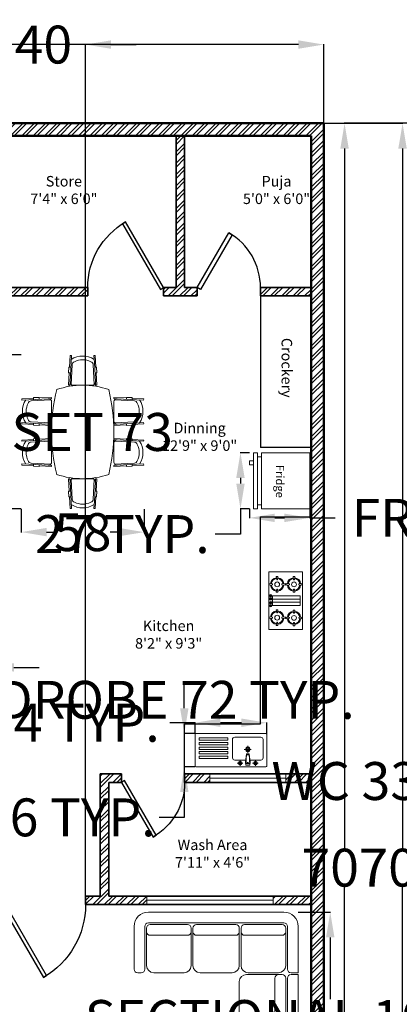
# Model space of a CAD drawing. Units: inches. Extents: x 73 to 1216, y -495 to 328.
# Tile 3 of 9: x 389 to 569, y -139 to 328. Entities that reach past the tile are written whole.
import ezdxf

# ---------------------------------------------------------------- set-up
doc = ezdxf.new("R2010")
doc.units = ezdxf.units.IN
for name, color, linetype, lineweight in [('A-ANNO-DIMS', 2, 'Continuous', 18), ('A-AREA-IDEN', 7, 'Continuous', 18), ('A-DOOR', 3, 'Continuous', 25), ('A-EQPM', 6, 'Continuous', 18), ('A-FLOR-FIXT', 9, 'Continuous', 18), ('A-GLAZ', 3, 'Continuous', 18), ('A-WALL-PATT', 8, 'Continuous', 13), ('Furniture', 2, 'Continuous', 18), ('Inner Walls', 5, 'Continuous', 35), ('Kitchen', 6, 'Continuous', 25), ('Outer Walls', 1, 'Continuous', 50), ('Text-T18', 7, 'Continuous', 18)]:
    doc.layers.add(name, color=color, linetype=linetype, lineweight=lineweight)
doc.styles.get("Standard").update_dxf_attribs({"font": 'arial.ttf'})
doc.dimstyles.get("Standard").update_dxf_attribs({"dimtxt": 18, "dimasz": 12, "dimexe": 0.18, "dimexo": 0.0625, "dimgap": 0.09, "dimtad": 0, "dimtih": 1, "dimtoh": 1, "dimdec": 0, "dimzin": 0, "dimdsep": 46, "dimlunit": 3, "dimtxsty": 'Standard', "dimcen": 0.09, "dimadec": 0, "dimazin": 0, "dimtfac": 1, "dimtdec": 0, "dimtofl": 0, "dimtmove": 0, "dimatfit": 3, "dimfxl": 1, "dimtolj": 1, "dimtzin": 0, "dimarcsym": 0})
pattern_1 = [(45, (-434.707, -1257.0093), (-2.694077, 2.694077), []), (45, (-432.911, -1257.0093), (-2.694077, 2.694077), [])]

# ---------------------------------------------------------------- blocks, each defined once
blk = doc.blocks.new('*U2')
for p, q in [((0, 0), (0, -4)), ((36, 0), (36, -4))]:
    blk.add_line(p, q)
blk.add_lwpolyline([(0, 0), (18, 31.18), (19.52, 30.3), (1.52, -0.88)], close=True)
blk.add_arc((0, 0), 36, 0, 60)
blk = doc.blocks.new('*U3')
for p, q in [((0, 0), (0, -4)), ((30, 0), (30, -4))]:
    blk.add_line(p, q)
blk.add_lwpolyline([(0, 0), (15, 25.98), (16.52, 25.11), (1.52, -0.88)], close=True)
blk.add_arc((0, 0), 30, 0, 60)
blk = doc.blocks.new('*U4')
for p, q in [((0, 0), (0, -4)), ((40, 0), (40, -4))]:
    blk.add_line(p, q)
blk.add_lwpolyline([(0, 0), (20, 34.64), (21.52, 33.77), (1.52, -0.88)], close=True)
blk.add_arc((0, 0), 40, 0, 60)
blk = doc.blocks.new('A$C6BEF12A9')
for p, q in [((0.698, 1.955), (0.688, 1.768)), ((0.698, 1.955), (0.718, 1.954)), ((0.718, 1.954), (0.712, 1.841)), ((1.099, 1.955), (1.079, 1.954)), ((1.079, 1.954), (1.085, 1.841)), ((1.099, 1.955), (1.109, 1.768)), ((1.358, 1.955), (1.349, 1.768)), ((1.358, 1.955), (1.378, 1.954)), ((1.378, 1.954), (1.372, 1.841)), ((1.76, 1.955), (1.74, 1.954)), ((1.74, 1.954), (1.746, 1.841)), ((1.76, 1.955), (1.77, 1.768)), ((0.678, 1.768), (0.673, 1.678)), ((0.708, 1.768), (0.678, 1.768)), ((0.712, 1.841), (0.695, 1.529)), ((0.712, 1.841), (0.695, 1.529)), ((0.73, 1.806), (0.713, 1.488)), ((1.067, 1.806), (1.084, 1.488)), ((1.085, 1.841), (1.102, 1.529)), ((1.089, 1.768), (1.119, 1.768)), ((1.119, 1.768), (1.124, 1.678)), ((1.339, 1.768), (1.334, 1.678)), ((1.369, 1.768), (1.339, 1.768)), ((1.372, 1.841), (1.356, 1.529)), ((1.372, 1.841), (1.356, 1.529)), ((1.391, 1.806), (1.374, 1.488)), ((1.728, 1.806), (1.744, 1.488)), ((1.746, 1.841), (1.762, 1.529)), ((1.75, 1.768), (1.78, 1.768)), ((1.78, 1.768), (1.784, 1.678)), ((0.683, 1.678), (0.673, 1.477)), ((0.703, 1.678), (0.673, 1.678)), ((1.094, 1.678), (1.124, 1.678)), ((1.114, 1.678), (1.124, 1.477)), ((1.344, 1.678), (1.333, 1.477)), ((1.364, 1.678), (1.334, 1.678)), ((1.754, 1.678), (1.784, 1.678)), ((1.774, 1.678), (1.785, 1.477)), ((0.673, 1.477), (0.693, 1.476)), ((0.693, 1.476), (0.695, 1.526)), ((0.745, 1.476), (1.052, 1.476)), ((1.104, 1.476), (1.102, 1.526)), ((1.124, 1.477), (1.104, 1.476)), ((1.333, 1.477), (1.353, 1.476)), ((1.353, 1.476), (1.356, 1.526)), ((1.406, 1.476), (1.712, 1.476)), ((1.765, 1.476), (1.762, 1.526)), ((1.785, 1.477), (1.765, 1.476)), ((0, 1.178), (0.187, 1.188)), ((0, 1.178), (0.001, 1.158)), ((0.001, 1.158), (0.114, 1.164)), ((0.114, 1.164), (0.426, 1.181)), ((0.149, 1.146), (0.467, 1.163)), ((0.187, 1.198), (0.277, 1.203)), ((0.187, 1.168), (0.187, 1.198)), ((0.277, 1.193), (0.477, 1.203)), ((0.277, 1.173), (0.277, 1.203)), ((0.479, 1.183), (0.429, 1.181)), ((0.477, 1.203), (0.479, 1.183)), ((0.479, 0.824), (0.479, 1.131)), ((1.98, 1.203), (1.979, 1.183)), ((1.979, 1.183), (2.029, 1.181)), ((1.979, 0.824), (1.979, 1.131)), ((2.18, 1.193), (1.98, 1.203)), ((2.309, 1.146), (1.99, 1.163)), ((2.343, 1.164), (2.031, 1.181)), ((2.18, 1.173), (2.18, 1.203)), ((2.27, 1.198), (2.18, 1.203)), ((2.27, 1.168), (2.27, 1.198)), ((2.458, 1.178), (2.27, 1.188)), ((2.457, 1.158), (2.343, 1.164)), ((2.458, 1.178), (2.457, 1.158)), ((0, 0.777), (0.001, 0.797)), ((0.001, 0.797), (0.114, 0.791)), ((0.114, 0.791), (0.426, 0.774)), ((0.114, 0.791), (0.426, 0.774)), ((0.149, 0.809), (0.467, 0.792)), ((2.309, 0.809), (1.99, 0.792)), ((2.343, 0.791), (2.031, 0.774)), ((2.343, 0.791), (2.031, 0.774)), ((2.457, 0.797), (2.343, 0.791)), ((2.458, 0.777), (2.457, 0.797)), ((0, 0.777), (0.187, 0.767)), ((0.187, 0.787), (0.187, 0.757)), ((0.187, 0.757), (0.277, 0.752)), ((0.277, 0.782), (0.277, 0.752)), ((0.277, 0.762), (0.477, 0.752)), ((0.479, 0.772), (0.429, 0.774)), ((0.477, 0.752), (0.479, 0.772)), ((1.979, 0.772), (2.029, 0.774)), ((1.98, 0.752), (1.979, 0.772)), ((2.18, 0.762), (1.98, 0.752)), ((2.18, 0.782), (2.18, 0.752)), ((2.27, 0.757), (2.18, 0.752)), ((2.27, 0.787), (2.27, 0.757)), ((2.458, 0.777), (2.27, 0.767)), ((0.673, 0.477), (0.693, 0.479)), ((0.683, 0.277), (0.673, 0.477)), ((0.693, 0.479), (0.695, 0.429)), ((0.745, 0.479), (1.052, 0.479)), ((1.104, 0.479), (1.102, 0.429)), ((1.124, 0.477), (1.104, 0.479)), ((1.114, 0.277), (1.124, 0.477)), ((1.333, 0.477), (1.353, 0.479)), ((1.344, 0.277), (1.333, 0.477)), ((1.353, 0.479), (1.356, 0.429)), ((1.406, 0.479), (1.712, 0.479)), ((1.765, 0.479), (1.762, 0.429)), ((1.785, 0.477), (1.765, 0.479)), ((1.774, 0.277), (1.785, 0.477)), ((0.712, 0.114), (0.695, 0.426)), ((0.712, 0.114), (0.695, 0.426)), ((0.73, 0.149), (0.713, 0.467)), ((1.067, 0.149), (1.084, 0.467)), ((1.085, 0.114), (1.102, 0.426)), ((1.372, 0.114), (1.356, 0.426)), ((1.372, 0.114), (1.356, 0.426)), ((1.391, 0.149), (1.374, 0.467)), ((1.728, 0.149), (1.744, 0.467)), ((1.746, 0.114), (1.762, 0.426)), ((0.678, 0.187), (0.673, 0.277)), ((0.703, 0.277), (0.673, 0.277)), ((0.708, 0.187), (0.678, 0.187)), ((0.698, 0), (0.688, 0.187)), ((1.089, 0.187), (1.119, 0.187)), ((1.094, 0.277), (1.124, 0.277)), ((1.099, 0), (1.109, 0.187)), ((1.119, 0.187), (1.124, 0.277)), ((1.364, 0.277), (1.334, 0.277)), ((1.339, 0.187), (1.334, 0.277)), ((1.369, 0.187), (1.339, 0.187)), ((1.358, 0), (1.349, 0.187)), ((1.75, 0.187), (1.78, 0.187)), ((1.754, 0.277), (1.784, 0.277)), ((1.76, 0), (1.77, 0.187)), ((1.78, 0.187), (1.784, 0.277)), ((0.698, 0), (0.718, 0.001)), ((0.718, 0.001), (0.712, 0.114)), ((1.079, 0.001), (1.085, 0.114)), ((1.099, 0), (1.079, 0.001)), ((1.358, 0), (1.378, 0.001)), ((1.378, 0.001), (1.372, 0.114)), ((1.74, 0.001), (1.746, 0.114)), ((1.76, 0), (1.74, 0.001))]:
    blk.add_line(p, q)
for centre, radius, start, end in [((0.898, 1.603), 0.341, 57.3412, 122.6588), ((1.559, 1.603), 0.341, 57.3412, 122.6588), ((0.78, 1.804), 0.05, 103.7138, 177), ((0.898, 1.603), 0.281, 62.3651, 117.6349), ((1.017, 1.804), 0.05, 3, 76.2862), ((1.441, 1.804), 0.05, 103.7138, 177), ((1.559, 1.603), 0.281, 62.3651, 117.6349), ((1.678, 1.804), 0.05, 3, 76.2862), ((1.229, -1.385), 2.862, 76.2365, 103.7635), ((0.745, 1.526), 0.05, 177, 270), ((1.052, 1.526), 0.05, 270, 3), ((1.406, 1.526), 0.05, 177, 270), ((1.712, 1.526), 0.05, 270, 3), ((1.779, 0.977), 1.3, 161.253, 198.747), ((0.679, 0.977), 1.3, 341.253, 18.747), ((0.352, 0.977), 0.341, 147.3412, 212.6588), ((0.352, 0.977), 0.281, 152.3651, 207.6349), ((0.151, 1.096), 0.05, 93, 166.2862), ((0.429, 1.131), 0.05, 0, 93), ((2.029, 1.131), 0.05, 87, 180), ((2.306, 1.096), 0.05, 13.7138, 87), ((2.106, 0.977), 0.281, 332.3651, 27.6349), ((2.106, 0.977), 0.341, 327.3412, 32.6588), ((0.151, 0.859), 0.05, 193.7138, 267), ((0.429, 0.824), 0.05, 267, 0), ((2.029, 0.824), 0.05, 180, 273), ((2.306, 0.859), 0.05, 273, 346.2862), ((1.229, 3.34), 2.862, 256.2365, 283.7635), ((0.745, 0.429), 0.05, 90, 183), ((1.052, 0.429), 0.05, 357, 90), ((1.406, 0.429), 0.05, 90, 183), ((1.712, 0.429), 0.05, 357, 90), ((0.898, 0.352), 0.341, 237.3412, 302.6588), ((0.78, 0.151), 0.05, 183, 256.2862), ((0.898, 0.352), 0.281, 242.3651, 297.6349), ((1.017, 0.151), 0.05, 283.7138, 357), ((1.559, 0.352), 0.341, 237.3412, 302.6588), ((1.441, 0.151), 0.05, 183, 256.2862), ((1.559, 0.352), 0.281, 242.3651, 297.6349), ((1.678, 0.151), 0.05, 283.7138, 357)]:
    blk.add_arc(centre, radius, start, end)
blk = doc.blocks.new('A$C2AFA021D')
for p, q in [((0.8, 2.3), (0.2, 2.3)), ((0.85, 2.2), (0.85, 2.25)), ((0, 2.1), (0, 0.2)), ((0.15, 0.2), (0.15, 2.1)), ((0.175, 1.55), (0.175, 2.075)), ((0.2, 2.15), (0.8, 2.15)), ((0.225, 2.125), (0.275, 2.125)), ((0.75, 2.125), (0.275, 2.125)), ((0.325, 2.075), (0.325, 1.55)), ((0.85, 1.6), (0.85, 2.025)), ((0.175, 0.875), (0.175, 1.425)), ((0.275, 1.5), (0.225, 1.5)), ((0.225, 1.475), (0.275, 1.475)), ((0.275, 1.5), (0.75, 1.5)), ((0.75, 1.475), (0.275, 1.475)), ((0.325, 1.425), (0.325, 0.875)), ((0.85, 0.925), (0.85, 1.375)), ((0.175, 0.225), (0.175, 0.75)), ((0.275, 0.825), (0.225, 0.825)), ((0.225, 0.8), (0.275, 0.8)), ((0.275, 0.825), (0.75, 0.825)), ((0.75, 0.8), (0.275, 0.8)), ((0.325, 0.75), (0.325, 0.225)), ((0.85, 0.275), (0.85, 0.7)), ((0.875, 0.275), (0.875, 0.725)), ((0.975, 0.825), (1.4, 0.825)), ((1.5, 0.725), (1.5, 0.275)), ((1.525, 0.275), (1.525, 0.725)), ((1.625, 0.825), (2.075, 0.825)), ((2.175, 0.725), (2.175, 0.275)), ((2.2, 0.275), (2.2, 0.725)), ((2.3, 0.825), (2.725, 0.825)), ((2.825, 0.725), (2.825, 0.275)), ((2.85, 0.2), (2.85, 0.775)), ((2.9, 0.825), (2.95, 0.825)), ((3, 0.775), (3, 0.2)), ((1.45, 0.325), (0.925, 0.325)), ((2.125, 0.325), (1.575, 0.325)), ((2.775, 0.325), (2.25, 0.325)), ((0.8, 0.15), (0.2, 0.15)), ((0.275, 0.175), (0.225, 0.175)), ((0.275, 0.175), (0.75, 0.175)), ((0.875, 0.275), (0.875, 0.225)), ((0.925, 0.175), (1.45, 0.175)), ((0.925, 0.15), (2.8, 0.15)), ((1.5, 0.225), (1.5, 0.275)), ((1.525, 0.275), (1.525, 0.225)), ((1.575, 0.175), (2.125, 0.175)), ((2.175, 0.225), (2.175, 0.275)), ((2.2, 0.275), (2.2, 0.225)), ((2.25, 0.175), (2.775, 0.175)), ((2.825, 0.225), (2.825, 0.275)), ((0.85, 0), (0.85, 0.1)), ((0.875, 0.1), (0.875, 0)), ((0.2, 0), (0.85, 0)), ((2.8, 0), (0.875, 0))]:
    blk.add_line(p, q)
for centre, radius, start, end in [((0.2, 2.1), 0.2, 90, 180), ((0.8, 2.25), 0.05, 0, 90), ((0.2, 2.1), 0.05, 90, 180), ((0.225, 2.075), 0.05, 90, 180), ((0.275, 2.075), 0.05, 0, 90), ((0.75, 2.025), 0.1, 0, 90), ((0.8, 2.2), 0.05, 270, 0), ((0.225, 1.55), 0.05, 180, 270), ((0.275, 1.55), 0.05, 270, 0), ((0.75, 1.6), 0.1, 270, 0), ((0.225, 1.425), 0.05, 90, 180), ((0.275, 1.425), 0.05, 0, 90), ((0.75, 1.375), 0.1, 360, 90), ((0.225, 0.875), 0.05, 180, 270), ((0.275, 0.875), 0.05, 270, 0), ((0.75, 0.925), 0.1, 270, 0), ((0.225, 0.75), 0.05, 90, 180), ((0.275, 0.75), 0.05, 0, 90), ((0.75, 0.7), 0.1, 0, 90), ((0.975, 0.725), 0.1, 90, 180), ((1.4, 0.725), 0.1, 0, 90), ((1.625, 0.725), 0.1, 90, 180), ((2.075, 0.725), 0.1, 0, 90), ((2.3, 0.725), 0.1, 90, 180), ((2.725, 0.725), 0.1, 0, 90), ((2.9, 0.775), 0.05, 90, 180), ((2.95, 0.775), 0.05, 0, 90), ((0.925, 0.275), 0.05, 90, 180), ((1.45, 0.275), 0.05, 360, 90), ((1.575, 0.275), 0.05, 90, 180), ((2.125, 0.275), 0.05, 360, 90), ((2.25, 0.275), 0.05, 90, 180), ((2.775, 0.275), 0.05, 360, 90), ((0.2, 0.2), 0.2, 180, 270), ((0.2, 0.2), 0.05, 180, 270), ((0.225, 0.225), 0.05, 180, 270), ((0.275, 0.225), 0.05, 270, 0), ((0.75, 0.275), 0.1, 270, 0), ((0.8, 0.1), 0.05, 0, 90), ((0.925, 0.225), 0.05, 180, 270), ((0.925, 0.1), 0.05, 90, 180), ((1.45, 0.225), 0.05, 270, 0), ((1.575, 0.225), 0.05, 180, 270), ((2.125, 0.225), 0.05, 270, 0), ((2.25, 0.225), 0.05, 180, 270), ((2.775, 0.225), 0.05, 270, 0), ((2.8, 0.2), 0.2, 270, 0), ((2.8, 0.2), 0.05, 270, 0)]:
    blk.add_arc(centre, radius, start, end)
blk = doc.blocks.new('REFRI-00')
for points in [[(-0.35, 0.35), (-0.35, -0.25), (0.35, -0.25), (0.35, 0.35), (-0.35, 0.35)], [(-0.35, -0.3), (-0.35, -0.35), (0.35, -0.35), (0.35, -0.3), (-0.35, -0.3)], [(-0.3, -0.3), (-0.3, -0.25)], [(-0.25, -0.35), (-0.25, -0.4), (-0.2, -0.4), (-0.2, -0.35)], [(0.3, -0.3), (0.3, -0.25)]]:
    blk.add_lwpolyline(points)
blk = doc.blocks.new('A$C57CF26DA')
for p, q in [((0, 0), (0, 420)), ((720, 420), (0, 420)), ((167, 413), (147, 413)), ((147, 413), (152, 373)), ((152, 373), (162, 373)), ((162, 373), (167, 413)), ((300, 391), (300, 49)), ((300, 391), (420, 391)), ((340, 391), (340, 49)), ((380, 391), (380, 49)), ((420, 391), (420, 49)), ((584, 413), (564, 413)), ((564, 413), (569, 373)), ((569, 373), (579, 373)), ((579, 373), (584, 413)), ((720, 0), (720, 420)), ((99, 320), (59, 325)), ((59, 325), (59, 305)), ((59, 305), (99, 310)), ((99, 310), (99, 320)), ((152, 257), (147, 217)), ((162, 257), (152, 257)), ((167, 217), (162, 257)), ((255, 325), (215, 320)), ((215, 320), (215, 310)), ((215, 310), (255, 305)), ((255, 305), (255, 325)), ((516, 320), (476, 325)), ((476, 325), (476, 305)), ((476, 305), (516, 310)), ((516, 310), (516, 320)), ((569, 257), (564, 217)), ((579, 257), (569, 257)), ((584, 217), (579, 257)), ((672, 325), (632, 320)), ((632, 320), (632, 310)), ((632, 310), (672, 305)), ((672, 305), (672, 325)), ((147, 217), (167, 217)), ((167, 203), (147, 203)), ((147, 203), (152, 163)), ((152, 163), (162, 163)), ((162, 163), (167, 203)), ((581, 203), (561, 203)), ((561, 203), (566, 163)), ((564, 217), (584, 217)), ((566, 163), (576, 163)), ((576, 163), (581, 203)), ((99, 110), (59, 115)), ((59, 115), (59, 95)), ((59, 95), (99, 100)), ((99, 100), (99, 110)), ((152, 47), (147, 7)), ((147, 7), (167, 7)), ((162, 47), (152, 47)), ((167, 7), (162, 47)), ((255, 115), (215, 110)), ((215, 110), (215, 100)), ((215, 100), (255, 95)), ((255, 95), (255, 115)), ((302, 39), (295, 39)), ((295, 39), (295, 11)), ((295, 11), (302, 11)), ((420, 49), (300, 49)), ((302, 11), (302, 39)), ((341, 39), (334, 39)), ((334, 39), (334, 11)), ((334, 11), (341, 11)), ((341, 11), (341, 39)), ((380, 11), (380, 39)), ((380, 39), (386, 39)), ((386, 11), (380, 11)), ((386, 39), (386, 11)), ((419, 11), (419, 39)), ((419, 39), (426, 39)), ((426, 11), (419, 11)), ((426, 39), (426, 11)), ((513, 110), (473, 115)), ((473, 115), (473, 95)), ((473, 95), (513, 100)), ((513, 100), (513, 110)), ((566, 47), (561, 7)), ((561, 7), (581, 7)), ((576, 47), (566, 47)), ((581, 7), (576, 47)), ((669, 115), (629, 110)), ((629, 110), (629, 100)), ((629, 100), (669, 95)), ((669, 95), (669, 115)), ((720, 0), (0, 0))]:
    blk.add_line(p, q)
for centre in [(157, 315), (574, 315), (157, 105), (571, 105)]:
    blk.add_circle(centre, 30)
for centre, radius, start, end in [((157, 315), 83, 95.5849, 174.4151), ((157, 315), 73, 95.3738, 174.6262), ((157, 315), 73, 5.3738, 84.6262), ((157, 315), 83, 5.5849, 84.4151), ((574, 315), 83, 95.5849, 174.4151), ((574, 315), 73, 95.3738, 174.6262), ((574, 315), 73, 5.3738, 84.6262), ((574, 315), 83, 5.5849, 84.4151), ((157, 315), 83, 185.5849, 264.4151), ((157, 315), 73, 185.3738, 264.6262), ((157, 315), 73, 275.3738, 354.6262), ((157, 315), 83, 275.5849, 354.4151), ((574, 315), 83, 185.5849, 264.4151), ((574, 315), 73, 185.3738, 264.6262), ((574, 315), 73, 275.3738, 354.6262), ((574, 315), 83, 275.5849, 354.4151), ((157, 105), 83, 95.5849, 174.4151), ((157, 105), 73, 95.3738, 174.6262), ((157, 105), 73, 5.3738, 84.6262), ((157, 105), 83, 5.5849, 84.4151), ((571, 105), 83, 95.5849, 174.4151), ((571, 105), 73, 95.3738, 174.6262), ((571, 105), 73, 5.3738, 84.6262), ((571, 105), 83, 5.5849, 84.4151), ((157, 105), 83, 185.5849, 264.4151), ((157, 105), 73, 185.3738, 264.6262), ((157, 105), 73, 275.3738, 354.6262), ((157, 105), 83, 275.5849, 354.4151), ((298, 25), 13.7, 104.4775, 255.5225), ((298, 25), 13.7, 284.4775, 75.5225), ((337, 25), 13.7, 104.4775, 255.5225), ((337, 25), 13.7, 284.4775, 75.5225), ((383, 25), 13.7, 104.4775, 255.5225), ((383, 25), 13.7, 284.4775, 75.5225), ((422, 25), 13.7, 104.4775, 255.5225), ((422, 25), 13.7, 284.4775, 75.5225), ((571, 105), 83, 185.5849, 264.4151), ((571, 105), 73, 185.3738, 264.6262), ((571, 105), 73, 275.3738, 354.6262), ((571, 105), 83, 275.5849, 354.4151)]:
    blk.add_arc(centre, radius, start, end)
blk = doc.blocks.new('A$C7C492201')
for p, q in [((0, 10), (0, 427)), ((10, 437), (927, 437)), ((112, 389), (185, 389)), ((148, 425), (148, 352)), ((223, 415), (217, 376)), ((223, 415), (232, 268)), ((223, 415), (248, 415)), ((225, 395), (248, 395)), ((273, 415), (248, 415)), ((272, 395), (248, 395)), ((273, 415), (265, 268)), ((273, 415), (280, 376)), ((312, 389), (385, 389)), ((348, 425), (348, 352)), ((937, 10), (937, 427)), ((48, 319), (48, 79)), ((221, 349), (78, 349)), ((217, 376), (232, 268)), ((231, 279), (248, 279)), ((232, 268), (248, 268)), ((266, 279), (248, 279)), ((265, 268), (248, 268)), ((280, 376), (265, 268)), ((418, 349), (276, 349)), ((448, 319), (448, 79)), ((509, 328), (509, 298)), ((509, 328), (885, 328)), ((509, 298), (885, 298)), ((509, 268), (509, 238)), ((509, 268), (885, 268)), ((885, 328), (885, 298)), ((885, 268), (885, 238)), ((203, 208), (294, 208)), ((248, 253), (248, 163)), ((509, 238), (885, 238)), ((509, 208), (885, 208)), ((509, 208), (509, 178)), ((509, 178), (885, 178)), ((509, 148), (509, 118)), ((509, 148), (885, 148)), ((885, 208), (885, 178)), ((885, 148), (885, 118)), ((927, 0), (10, 0)), ((418, 49), (78, 49)), ((509, 118), (885, 118)), ((509, 88), (509, 58)), ((509, 88), (885, 88)), ((509, 58), (885, 58)), ((885, 88), (885, 58))]:
    blk.add_line(p, q)
for centre, radius in [((148, 389), 25), ((148, 389), 15), ((348, 389), 25), ((348, 389), 15), ((248, 208), 30), ((248, 208), 20)]:
    blk.add_circle(centre, radius)
for centre, radius, start, end in [((10, 427), 10, 90, 180), ((247, 388), 7.19, 80.5252, 279.4748), ((250, 388), 7.19, 260.5252, 99.4748), ((927, 427), 10, 0, 90), ((78, 319), 30, 90, 180), ((418, 319), 30, 0, 90), ((10, 10), 10, 180, 270), ((78, 79), 30, 180, 270), ((418, 79), 30, 270, 0), ((927, 10), 10, 270, 0)]:
    blk.add_arc(centre, radius, start, end)
blk = doc.blocks.new('*U19')
for p, q in [((0, 4), (0, 0)), ((0, 2), (36, 2)), ((36, 4), (36, 0))]:
    blk.add_line(p, q)
blk = doc.blocks.new('*U20')
for p, q in [((0, 4), (0, 0)), ((0, 2), (60, 2)), ((60, 4), (60, 0))]:
    blk.add_line(p, q)
blk = doc.blocks.new('*D28')
at = {"layer": 'A-ANNO-DIMS', "color": 0, "lineweight": -2, "transparency": 16777216}
for p, q in [((520.8, -95.45), (536.15, -95.45)), ((535.97, -107.45), (535.97, -136.81)), ((535.97, -184.97), (535.97, -155.61)), ((520.8, -196.97), (536.15, -196.97))]:
    blk.add_line(p, q, dxfattribs=at)
at = {"layer": 'A-ANNO-DIMS', "color": 0, "transparency": 16777216}
for points in [[(533.97, -107.45), (537.97, -107.45), (535.97, -95.45)], [(533.97, -184.97), (537.97, -184.97), (535.97, -196.97)]]:
    blk.add_solid(points, dxfattribs=at)
at = {"layer": 'Defpoints', "color": 0, "transparency": 16777216}
for p in [(520.74, -95.45), (520.74, -196.97), (535.97, -196.97)]:
    blk.add_point(p, dxfattribs=at)
at = {"layer": 'A-ANNO-DIMS', "color": 0, "transparency": 16777216, "insert": (535.97, -146.21), "char_height": 18, "attachment_point": 5}
blk.add_mtext('\\A1;SECTIONAL 102 TYP.', dxfattribs=at)
blk = doc.blocks.new('*D30')
at = {"layer": 'A-ANNO-DIMS', "color": 0, "lineweight": -2, "transparency": 16777216}
for p, q in [((656.55, 12.18), (651.43, 12.18)), ((651.61, 0.18), (651.61, -9.18)), ((656.55, -21.18), (651.43, -21.18)), ((651.61, -21.18), (651.61, -33.18)), ((651.61, -33.18), (639.61, -33.18))]:
    blk.add_line(p, q, dxfattribs=at)
at = {"layer": 'A-ANNO-DIMS', "color": 0, "transparency": 16777216}
for points in [[(649.61, 0.18), (653.61, 0.18), (651.61, 12.18)], [(649.61, -9.18), (653.61, -9.18), (651.61, -21.18)]]:
    blk.add_solid(points, dxfattribs=at)
at = {"layer": 'Defpoints', "color": 0, "transparency": 16777216}
for p in [(656.61, 12.18), (651.61, -21.18), (656.61, -21.18)]:
    blk.add_point(p, dxfattribs=at)
at = {"layer": 'A-ANNO-DIMS', "color": 0, "transparency": 16777216, "insert": (570.9, -33.18), "char_height": 18, "attachment_point": 5}
blk.add_mtext('\\A1;WC 33 TYP.', dxfattribs=at)
blk = doc.blocks.new('*D36')
at = {"layer": 'A-ANNO-DIMS', "color": 0, "lineweight": -2, "transparency": 16777216}
for p, q in [((230.87, 16.11), (230.87, 5.2)), ((302.87, 16.11), (302.87, 5.2)), ((242.87, 5.38), (290.87, 5.38)), ((302.87, 5.38), (314.87, 5.38))]:
    blk.add_line(p, q, dxfattribs=at)
at = {"layer": 'A-ANNO-DIMS', "color": 0, "transparency": 16777216}
for points in [[(242.87, 7.38), (242.87, 3.38), (230.87, 5.38)], [(290.87, 7.38), (290.87, 3.38), (302.87, 5.38)]]:
    blk.add_solid(points, dxfattribs=at)
at = {"layer": 'Defpoints', "color": 0, "transparency": 16777216}
for p in [(230.87, 16.18), (302.87, 16.18), (302.87, 5.38)]:
    blk.add_point(p, dxfattribs=at)
at = {"layer": 'A-ANNO-DIMS', "color": 0, "transparency": 16777216, "insert": (436.68, 5.38), "char_height": 18, "attachment_point": 5}
blk.add_mtext('\\A1;WARDROBE 72 TYP.', dxfattribs=at)
blk = doc.blocks.new('*D40')
at = {"layer": 'A-ANNO-DIMS', "color": 0, "lineweight": -2, "transparency": 16777216}
for p, q in [((497.66, 96.03), (497.66, 91.62)), ((526.23, 96.03), (526.23, 91.62)), ((509.66, 91.8), (514.23, 91.8)), ((526.23, 91.8), (538.23, 91.8))]:
    blk.add_line(p, q, dxfattribs=at)
at = {"layer": 'A-ANNO-DIMS', "color": 0, "transparency": 16777216}
for points in [[(509.66, 93.8), (509.66, 89.8), (497.66, 91.8)], [(514.23, 93.8), (514.23, 89.8), (526.23, 91.8)]]:
    blk.add_solid(points, dxfattribs=at)
at = {"layer": 'Defpoints', "color": 0, "transparency": 16777216}
for p in [(497.66, 96.09), (526.23, 96.09), (526.23, 91.8)]:
    blk.add_point(p, dxfattribs=at)
at = {"layer": 'A-ANNO-DIMS', "color": 0, "transparency": 16777216, "insert": (632.61, 91.8), "char_height": 18, "attachment_point": 5}
blk.add_mtext('\\A1;FRIDGE 29 TYP.', dxfattribs=at)
blk = doc.blocks.new('*D41')
at = {"layer": 'A-ANNO-DIMS', "color": 0, "lineweight": -2, "transparency": 16777216}
for p, q in [((497.6, 122.75), (493.19, 122.75)), ((493.37, 110.75), (493.37, 108.09)), ((497.6, 96.09), (493.19, 96.09)), ((493.37, 96.09), (493.37, 84.09)), ((493.37, 84.09), (481.37, 84.09))]:
    blk.add_line(p, q, dxfattribs=at)
at = {"layer": 'A-ANNO-DIMS', "color": 0, "transparency": 16777216}
for points in [[(491.37, 110.75), (495.37, 110.75), (493.37, 122.75)], [(491.37, 108.09), (495.37, 108.09), (493.37, 96.09)]]:
    blk.add_solid(points, dxfattribs=at)
at = {"layer": 'Defpoints', "color": 0, "transparency": 16777216}
for p in [(497.66, 122.75), (493.37, 96.09), (497.66, 96.09)]:
    blk.add_point(p, dxfattribs=at)
at = {"layer": 'A-ANNO-DIMS', "color": 0, "transparency": 16777216, "insert": (437.32, 84.09), "char_height": 18, "attachment_point": 5}
blk.add_mtext('\\A1;27 TYP.', dxfattribs=at)
blk = doc.blocks.new('*D44')
at = {"layer": 'A-ANNO-DIMS', "color": 0, "lineweight": -2, "transparency": 16777216}
for p, q in [((471.83, -5.5), (459.83, -5.5)), ((471.83, -10.54), (471.83, -5.32)), ((493.84, -5.5), (483.83, -5.5)), ((505.84, -10.54), (505.84, -5.32))]:
    blk.add_line(p, q, dxfattribs=at)
at = {"layer": 'A-ANNO-DIMS', "color": 0, "transparency": 16777216}
for points in [[(483.83, -3.5), (483.83, -7.5), (471.83, -5.5)], [(493.84, -3.5), (493.84, -7.5), (505.84, -5.5)]]:
    blk.add_solid(points, dxfattribs=at)
at = {"layer": 'Defpoints', "color": 0, "transparency": 16777216}
for p in [(471.83, -5.5), (471.83, -10.6), (505.84, -10.6)]:
    blk.add_point(p, dxfattribs=at)
at = {"layer": 'A-ANNO-DIMS', "color": 0, "transparency": 16777216, "insert": (383.14, -5.5), "char_height": 18, "attachment_point": 5}
blk.add_mtext('\\A1;SINK 34 TYP.', dxfattribs=at)
blk = doc.blocks.new('*D45')
at = {"layer": 'A-ANNO-DIMS', "color": 0, "lineweight": -2, "transparency": 16777216}
for p, q in [((466.73, 1.4), (466.73, 13.4)), ((471.77, -10.6), (466.55, -10.6)), ((471.77, -26.44), (466.55, -26.44)), ((466.73, -38.44), (466.73, -50.44)), ((466.73, -50.44), (454.73, -50.44))]:
    blk.add_line(p, q, dxfattribs=at)
at = {"layer": 'A-ANNO-DIMS', "color": 0, "transparency": 16777216}
for points in [[(464.73, 1.4), (468.73, 1.4), (466.73, -10.6)], [(464.73, -38.44), (468.73, -38.44), (466.73, -26.44)]]:
    blk.add_solid(points, dxfattribs=at)
at = {"layer": 'Defpoints', "color": 0, "transparency": 16777216}
for p in [(471.83, -10.6), (466.73, -26.44), (471.83, -26.44)]:
    blk.add_point(p, dxfattribs=at)
at = {"layer": 'A-ANNO-DIMS', "color": 0, "transparency": 16777216, "insert": (411.68, -50.44), "char_height": 18, "attachment_point": 5}
blk.add_mtext('\\A1;16 TYP.', dxfattribs=at)
blk = doc.blocks.new('*D48')
at = {"layer": 'A-ANNO-DIMS', "color": 0, "lineweight": -2, "transparency": 16777216}
for p, q in [((389.31, 169.17), (378.22, 169.17)), ((378.4, 157.17), (378.4, 141.99)), ((378.4, 108.01), (378.4, 123.19)), ((389.31, 96.01), (378.22, 96.01))]:
    blk.add_line(p, q, dxfattribs=at)
at = {"layer": 'A-ANNO-DIMS', "color": 0, "transparency": 16777216}
for points in [[(376.4, 157.17), (380.4, 157.17), (378.4, 169.17)], [(376.4, 108.01), (380.4, 108.01), (378.4, 96.01)]]:
    blk.add_solid(points, dxfattribs=at)
at = {"layer": 'Defpoints', "color": 0, "transparency": 16777216}
for p in [(389.37, 169.17), (378.4, 96.01), (389.37, 96.01)]:
    blk.add_point(p, dxfattribs=at)
at = {"layer": 'A-ANNO-DIMS', "color": 0, "transparency": 16777216, "insert": (378.4, 132.59), "char_height": 18, "attachment_point": 5}
blk.add_mtext('\\A1;DINING SET 73', dxfattribs=at)
blk = doc.blocks.new('*D49')
at = {"layer": 'A-ANNO-DIMS', "color": 0, "lineweight": -2, "transparency": 16777216}
for p, q in [((389.37, 95.95), (389.37, 84.85)), ((447.66, 95.95), (447.66, 84.85)), ((401.37, 85.03), (405.51, 85.03)), ((435.66, 85.03), (431.52, 85.03))]:
    blk.add_line(p, q, dxfattribs=at)
at = {"layer": 'A-ANNO-DIMS', "color": 0, "transparency": 16777216}
for points in [[(401.37, 87.03), (401.37, 83.03), (389.37, 85.03)], [(435.66, 87.03), (435.66, 83.03), (447.66, 85.03)]]:
    blk.add_solid(points, dxfattribs=at)
at = {"layer": 'Defpoints', "color": 0, "transparency": 16777216}
for p in [(389.37, 96.01), (447.66, 96.01), (447.66, 85.03)]:
    blk.add_point(p, dxfattribs=at)
at = {"layer": 'A-ANNO-DIMS', "color": 0, "transparency": 16777216, "insert": (418.52, 85.03), "char_height": 18, "attachment_point": 5}
blk.add_mtext('\\A1;58', dxfattribs=at)
blk = doc.blocks.new('*D50')
at = {"layer": 'A-ANNO-DIMS', "color": 0, "lineweight": -2, "transparency": 16777216}
for p, q in [((182.87, 279.24), (182.87, 316.76)), ((194.87, 316.58), (337.94, 316.58)), ((520.87, 316.58), (377.81, 316.58)), ((532.87, 279.24), (532.87, 316.76))]:
    blk.add_line(p, q, dxfattribs=at)
at = {"layer": 'A-ANNO-DIMS', "color": 0, "transparency": 16777216}
for points in [[(194.87, 318.58), (194.87, 314.58), (182.87, 316.58)], [(520.87, 318.58), (520.87, 314.58), (532.87, 316.58)]]:
    blk.add_solid(points, dxfattribs=at)
at = {"layer": 'Defpoints', "color": 0, "transparency": 16777216}
for p in [(532.87, 316.58), (182.87, 279.18), (532.87, 279.18)]:
    blk.add_point(p, dxfattribs=at)
at = {"layer": 'A-ANNO-DIMS', "color": 0, "transparency": 16777216, "insert": (357.87, 316.58), "char_height": 18, "attachment_point": 5}
blk.add_mtext('\\A1;350', dxfattribs=at)
blk = doc.blocks.new('*D51')
at = {"layer": 'A-ANNO-DIMS', "color": 0, "lineweight": -2, "transparency": 16777216}
for p, q in [((532.94, 279.18), (570.45, 279.18)), ((570.27, 267.18), (570.27, -65.04)), ((570.27, -415.82), (570.27, -83.6)), ((532.94, -427.82), (570.45, -427.82))]:
    blk.add_line(p, q, dxfattribs=at)
at = {"layer": 'A-ANNO-DIMS', "color": 0, "transparency": 16777216}
for points in [[(568.27, 267.18), (572.27, 267.18), (570.27, 279.18)], [(568.27, -415.82), (572.27, -415.82), (570.27, -427.82)]]:
    blk.add_solid(points, dxfattribs=at)
at = {"layer": 'Defpoints', "color": 0, "transparency": 16777216}
for p in [(532.87, 279.18), (570.27, 279.18), (532.87, -427.82)]:
    blk.add_point(p, dxfattribs=at)
at = {"layer": 'A-ANNO-DIMS', "color": 0, "transparency": 16777216, "insert": (570.27, -74.32), "char_height": 18, "attachment_point": 5}
blk.add_mtext('\\A1;707', dxfattribs=at)
blk = doc.blocks.new('*D53')
at = {"layer": 'A-ANNO-DIMS', "color": 0, "lineweight": -2, "transparency": 16777216}
for p, q in [((580.1, 279.18), (542.58, 279.18)), ((542.76, 267.18), (542.76, -65.04)), ((542.76, -415.82), (542.76, -83.6)), ((580.1, -427.82), (542.58, -427.82))]:
    blk.add_line(p, q, dxfattribs=at)
at = {"layer": 'A-ANNO-DIMS', "color": 0, "transparency": 16777216}
for points in [[(540.76, 267.18), (544.76, 267.18), (542.76, 279.18)], [(540.76, -415.82), (544.76, -415.82), (542.76, -427.82)]]:
    blk.add_solid(points, dxfattribs=at)
at = {"layer": 'Defpoints', "color": 0, "transparency": 16777216}
for p in [(542.76, 279.18), (580.16, 279.18), (580.16, -427.82)]:
    blk.add_point(p, dxfattribs=at)
at = {"layer": 'A-ANNO-DIMS', "color": 0, "transparency": 16777216, "insert": (542.76, -74.32), "char_height": 18, "attachment_point": 5}
blk.add_mtext('\\A1;707', dxfattribs=at)
blk = doc.blocks.new('*D62')
at = {"layer": 'A-ANNO-DIMS', "color": 0, "lineweight": -2, "transparency": 16777216}
for p, q in [((367.87461, 316.576301), (355.87461, 316.576301)), ((379.87461, -87.761199), (379.87461, 316.756301)), ((419.87461, -87.761199), (419.87461, 316.756301)), ((431.87461, 316.576301), (443.87461, 316.576301))]:
    blk.add_line(p, q, dxfattribs=at)
at = {"layer": 'A-ANNO-DIMS', "color": 0, "transparency": 16777216}
for points in [[(367.87461, 318.576301), (367.87461, 314.576301), (379.87461, 316.576301)], [(431.87461, 318.576301), (431.87461, 314.576301), (419.87461, 316.576301)]]:
    blk.add_solid(points, dxfattribs=at)
at = {"layer": 'Defpoints', "color": 0, "transparency": 16777216}
for p in [(419.87461, 316.576301), (379.87461, -87.823699), (419.87461, -87.823699)]:
    blk.add_point(p, dxfattribs=at)
at = {"layer": 'A-ANNO-DIMS', "color": 0, "transparency": 16777216, "insert": (399.87461, 316.576301), "char_height": 18, "attachment_point": 5}
blk.add_mtext('\\A1;40', dxfattribs=at)
blk = doc.blocks.new('*D71')
at = {"layer": 'A-ANNO-DIMS', "color": 0, "lineweight": -2, "transparency": 16777216}
for p, q in [((369.87, 58.11), (369.87, 20.6)), ((373.87, 58.11), (373.87, 20.6)), ((357.87, 20.78), (345.87, 20.78)), ((385.87, 20.78), (397.87, 20.78))]:
    blk.add_line(p, q, dxfattribs=at)
at = {"layer": 'A-ANNO-DIMS', "color": 0, "transparency": 16777216}
for points in [[(357.87, 22.78), (357.87, 18.78), (369.87, 20.78)], [(385.87, 22.78), (385.87, 18.78), (373.87, 20.78)]]:
    blk.add_solid(points, dxfattribs=at)
at = {"layer": 'Defpoints', "color": 0, "transparency": 16777216}
for p in [(369.87, 58.18), (373.87, 58.18), (369.87, 20.78)]:
    blk.add_point(p, dxfattribs=at)
at = {"layer": 'A-ANNO-DIMS', "color": 0, "transparency": 16777216, "insert": (339.56, 20.78), "char_height": 18, "attachment_point": 5}
blk.add_mtext('\\A1;4', dxfattribs=at)

msp = doc.modelspace()

# ---------------------------------------------------------------- hatches: boundary and pattern name
at = {"layer": 'A-WALL-PATT'}
h = msp.add_hatch(dxfattribs=at)
h.set_pattern_fill('ANSI32', color=256, scale=0.4)
h.set_pattern_definition(pattern_1)
h.paths.add_polyline_path([(526.8746, -307.8237), (365.8746, -307.8237), (365.8746, -421.8237), (369.8746, -421.8237), (369.8746, -313.8237), (526.8746, -313.8237)], flags=17)
h.paths.add_polyline_path([(532.8746, 279.1763), (182.8746, 279.1763), (182.8746, -427.8237), (235.8746, -427.8237), (235.8746, -421.8237), (188.8746, -421.8237), (188.8746, 273.1763), (526.8746, 273.1763), (526.8746, -421.8237), (355.8746, -421.8237), (355.8746, -427.8237), (532.8746, -427.8237)])
h.paths.add_polyline_path([(230.8746, 197.1763), (224.8746, 197.1763), (224.8746, 83.4706), (230.8746, 83.4706)], flags=17)
h = msp.add_hatch(dxfattribs=at)
h.set_pattern_fill('ANSI32', color=256, scale=0.4)
h.set_pattern_definition(pattern_1)
h.paths.add_polyline_path([(287.8746, 201.1763), (281.8746, 201.1763), (281.8746, 206.1763), (277.8746, 206.1763), (277.8746, 201.1763), (218.9775, 201.1763), (218.9775, 197.1763), (287.8746, 197.1763)])
h.paths.add_polyline_path([(194.9775, 201.1763), (188.8746, 201.1763), (188.8746, 197.1763), (194.9775, 197.1763)])
h.paths.add_polyline_path([(281.8746, 273.1763), (277.8746, 273.1763), (277.8746, 236.1763), (281.8746, 236.1763)])
h.paths.add_polyline_path([(420.8746, 201.1763), (374.8746, 201.1763), (374.8746, 273.1763), (370.8746, 273.1763), (370.8746, 249.1763), (370.8746, 201.1763), (323.8746, 201.1763), (323.8746, 197.1763), (369.8746, 197.1763), (369.8746, 58.1763), (373.8746, 58.1763), (373.8746, 197.1763), (420.8746, 197.1763)])
h.paths.add_polyline_path([(472.8746, 201.1763), (466.8746, 201.1763), (466.8746, 273.1763), (462.8746, 273.1763), (462.8746, 201.1763), (456.8746, 201.1763), (456.8746, 197.1763), (472.8746, 197.1763)])
h.paths.add_polyline_path([(526.8746, 201.1763), (502.8746, 201.1763), (502.8746, 197.1763), (526.8746, 197.1763)])
h.paths.add_polyline_path([(373.8746, 22.1763), (369.8746, 22.1763), (369.8746, 16.1763), (230.8746, 16.1763), (230.8746, 12.1763), (373.8746, 12.1763)])
h.paths.add_polyline_path([(318.8746, -17.8237), (230.8746, -17.8237), (230.8746, -21.8237), (314.8746, -21.8237), (314.8746, -27.8237), (318.8746, -27.8237)])
h.paths.add_polyline_path([(327.8746, -87.8237), (318.8746, -87.8237), (318.8746, -57.8237), (314.8746, -57.8237), (314.8746, -87.8237), (230.8746, -87.8237), (230.8746, -91.8237), (327.8746, -91.8237)])
h.paths.add_polyline_path([(379.8746, -87.8237), (363.8746, -87.8237), (363.8746, -91.8237), (369.8746, -91.8237), (369.8746, -223.8237), (373.8746, -223.8237), (373.8746, -91.8237), (379.8746, -91.8237)])
h.paths.add_polyline_path([(448.8746, -87.8237), (430.8746, -87.8237), (430.8746, -33.8237), (436.8746, -33.8237), (436.8746, -29.8237), (426.8746, -29.8237), (426.8746, -87.8237), (419.8746, -87.8237), (419.8746, -91.8237), (448.8746, -91.8237)])
h.paths.add_polyline_path([(526.8746, -87.8237), (508.8746, -87.8237), (508.8746, -91.8237), (526.8746, -91.8237)])
h.paths.add_polyline_path([(526.8746, -29.8237), (514.8746, -29.8237), (514.8746, -33.8237), (526.8746, -33.8237)])
h.paths.add_polyline_path([(478.8746, -29.8237), (466.8746, -29.8237), (466.8746, -33.8237), (478.8746, -33.8237)])

# ---------------------------------------------------------------- linework, layer by layer
at = {"layer": 'Inner Walls'}
for p, q in [((462.8746, 273.1763), (462.8746, 201.1763)), ((466.8746, 273.1763), (466.8746, 201.1763)), ((420.8746, 201.1763), (374.8746, 201.1763)), ((420.8746, 197.1763), (420.8746, 201.1763)), ((462.8746, 201.1763), (456.8746, 201.1763)), ((456.8746, 201.1763), (456.8746, 197.1763)), ((472.8746, 201.1763), (466.8746, 201.1763)), ((472.8746, 201.1763), (472.8746, 197.1763)), ((526.8746, 201.1763), (502.8746, 201.1763)), ((502.8746, 197.1763), (502.8746, 201.1763)), ((420.8746, 197.1763), (373.8746, 197.1763)), ((472.8746, 197.1763), (456.8746, 197.1763)), ((526.8746, 197.1763), (502.8746, 197.1763)), ((426.8746, -87.8237), (426.8746, -29.8237)), ((436.8746, -29.8237), (426.8746, -29.8237)), ((436.8746, -33.8237), (436.8746, -29.8237)), ((526.8746, -29.8237), (466.8746, -29.8237)), ((466.8746, -29.8237), (466.8746, -33.8237)), ((430.8746, -87.8237), (430.8746, -33.8237)), ((436.8746, -33.8237), (430.8746, -33.8237)), ((526.8746, -33.8237), (466.8746, -33.8237)), ((426.8746, -87.8237), (419.8746, -87.8237)), ((419.8746, -87.8237), (419.8746, -91.8237)), ((526.8746, -87.8237), (430.8746, -87.8237)), ((526.8746, -91.8237), (419.8746, -91.8237))]:
    msp.add_line(p, q, dxfattribs=at)
at = {"layer": 'Kitchen'}
for p, q in [((526.8746, 197.1763), (502.8746, 197.1763)), ((502.8746, 197.1763), (502.8746, 125.1763)), ((526.8746, 125.1763), (502.8746, 125.1763))]:
    msp.add_line(p, q, dxfattribs=at)
msp.add_lwpolyline([(466.8746, -6.0549), (502.8746, -6.0549), (502.8746, 92.3336), (526.8746, 92.3336), (526.8746, -29.8237), (466.8746, -29.8237)], close=True, dxfattribs=at)
at = {"layer": 'Outer Walls'}
for p, q in [((182.8746, 279.1763), (532.8746, 279.1763)), ((532.8746, -427.8237), (532.8746, 279.1763)), ((188.8746, 273.1763), (526.8746, 273.1763)), ((526.8746, -421.8237), (526.8746, 273.1763))]:
    msp.add_line(p, q, dxfattribs=at)

# ---------------------------------------------------------------- block references
at = {"layer": 'A-DOOR', "xscale": -1}
msp.add_blockref('*U2', (456.8746, 201.1763), dxfattribs=at)
at = {"layer": 'A-DOOR'}
msp.add_blockref('*U3', (472.8746, 201.1763), dxfattribs=at)
at = {"layer": 'A-DOOR', "xscale": -1, "rotation": 180}
for name, p in [('*U3', (436.8746, -33.8237)), ('*U4', (379.8746, -91.8237))]:
    msp.add_blockref(name, p, dxfattribs=at)
at = {"layer": 'A-EQPM', "rotation": 270}
for name, p, xscale, yscale, zscale in [('REFRI-00', (512.8968, 109.4204), 38.0932829071003, 38.0932829071003, 38.0932829071003), ('A$C57CF26DA', (506.7572, 66.2039), 0.0381707681172169, 0.0381707681172169, 0.0381707681172169)]:
    msp.add_blockref(name, p, dxfattribs=dict(at, xscale=xscale, yscale=yscale, zscale=zscale))
at = {"layer": 'A-FLOR-FIXT', "xscale": 0.0362851414289068, "yscale": 0.0362851414289068, "zscale": 0.0362851414289068, "rotation": 180}
msp.add_blockref('A$C7C492201', (505.8405, -10.5999), dxfattribs=at)
at = {"layer": 'A-GLAZ'}
for name, p in [('*U19', (478.8746, -33.8237)), ('*U20', (448.8746, -91.8237))]:
    msp.add_blockref(name, p, dxfattribs=at)
at = {"layer": 'Furniture'}
for name, p, xscale, yscale, zscale, rotation in [('A$C6BEF12A9', (389.5901, 168.9515), 29.59247402267948, 29.59247402267948, 29.59247402267948, 270), ('A$C2AFA021D', (520.7411, -95.4493), -33.84012530478223, 33.84012530478223, 33.84012530478223, 90)]:
    msp.add_blockref(name, p, dxfattribs=dict(at, xscale=xscale, yscale=yscale, zscale=zscale, rotation=rotation))

# ---------------------------------------------------------------- texts
at = {"layer": 'A-AREA-IDEN', "char_height": 5, "attachment_point": 3}
for s, width, insert in [('\\pxqc;{\\fTimes New Roman|b0|i0|c0|p18;Store\\P7\'4" x 6\'0"}', 37.203385, (428.1814, 254.167)), ('\\pxqc;{\\fTimes New Roman|b0|i0|c0|p18;Puja\\P5\'0" x 6\'0"}', 37.203385, (529.0816, 254.167)), ('\\pxqc;{\\fTimes New Roman|b0|i0|c0|p18;Dinning\\P12\'9" x 9\'0"}', 37.203385, (492.6014, 136.9478)), ('\\pxqc;{\\fTimes New Roman|b0|i0|c0|p18;Kitchen\\P8\'2" x 9\'3"}', 49.101878, (483.8367, 43.0375)), ('\\pxqc;{\\fTimes New Roman|b0|i0|c0|p18;Wash Area\\P7\'11" x 4\'6"}', 49.101878, (504.6592, -60.9763))]:
    msp.add_mtext_dynamic_manual_height_columns(s, width=width, gutter_width=12.5, heights=[0], dxfattribs=dict(at, insert=insert))
at = {"layer": 'Text-T18', "rotation": 270}
for s, width, gutter_width, insert, char_height, attachment_point in [('\\pxqc;{\\fTimes New Roman|b0|i0|c0|p18;Crockery}', 37.203385, 12.5, (517.8774, 144.4874), 5, 3), ('\\pxqc;{\\fTimes New Roman|b0|i0|c0|p18;Fridge}', 17.951771, 4.8475, (514.0796, 118.0951), 3.877971, 1)]:
    msp.add_mtext_dynamic_manual_height_columns(s, width=width, gutter_width=gutter_width, heights=[0], dxfattribs=dict(at, insert=insert, char_height=char_height, attachment_point=attachment_point))

# ---------------------------------------------------------------- dimensions: what is measured, and where the dimension line sits
at = {"layer": 'A-ANNO-DIMS'}
for base, p1, p2, picture, middle in [((532.8746, 316.5763), (182.8746, 279.1763), (532.8746, 279.1763), '*D50', (357.8746, 316.5763)), ((419.8746, 316.5763), (379.8746, -87.8237), (419.8746, -87.8237), '*D62', (399.8746, 316.5763)), ((447.6584, 85.0341), (389.3726, 96.0082), (447.6584, 96.0082), '*D49', (418.5155, 85.0341))]:
    dim = msp.add_linear_dim(base=base, p1=p1, p2=p2, dimstyle='Standard', override={"dimdec": 0, "dimlfac": 1, "dimrnd": 0, "dimzin": 0, "dimdsep": 46, "dimlunit": 2}, dxfattribs=at)
    dim.commit()
    dim.dimension.update_dxf_attribs({"geometry": picture, "text_midpoint": middle})
for base, p1, p2, angle, picture, middle in [((542.7647, 279.1763), (580.1647, -427.8237), (580.1647, 279.1763), 90, '*D53', (542.7647, -74.3237)), ((570.2746, 279.1763), (532.8746, -427.8237), (532.8746, 279.1763), 90, '*D51', (570.2746, -74.3237)), ((369.8746, 20.7763), (373.8746, 58.1763), (369.8746, 58.1763), 180, '*D71', (339.5595, 20.7763))]:
    dim = msp.add_linear_dim(base=base, p1=p1, p2=p2, angle=angle, dimstyle='Standard', override={"dimdec": 0, "dimlfac": 1, "dimrnd": 0, "dimzin": 0, "dimdsep": 46, "dimlunit": 2}, dxfattribs=at)
    dim.commit()
    dim.dimension.update_dxf_attribs({"geometry": picture, "text_midpoint": middle})
for base, p1, p2, angle, text, picture, middle in [((378.3985, 96.0082), (389.3726, 169.169), (389.3726, 96.0082), 270, 'DINING SET <>', '*D48', (378.3985, 132.5886)), ((493.374, 96.0877), (497.6595, 122.753), (497.6595, 96.0877), 270, '<> TYP.', '*D41', (437.3215, 84.0877)), ((471.8322, -5.4987), (505.8405, -10.5999), (471.8322, -10.5999), 180, 'SINK <> TYP.', '*D44', (383.1378, -5.4987)), ((466.7309, -26.4423), (471.8322, -10.5999), (471.8322, -26.4423), 270, '<> TYP.', '*D45', (411.6791, -50.4423)), ((651.6053, -21.1805), (656.6088, 12.1763), (656.6088, -21.1805), 270, 'WC <> TYP.', '*D30', (570.898, -33.1805)), ((535.9692, -196.9696), (520.7411, -95.4493), (520.7411, -196.9696), 270, 'SECTIONAL <> TYP.', '*D28', (535.9692, -146.2095))]:
    dim = msp.add_linear_dim(base=base, p1=p1, p2=p2, angle=angle, text=text, dimstyle='Standard', override={"dimdec": 0, "dimlfac": 1, "dimrnd": 0, "dimzin": 0, "dimdsep": 46, "dimlunit": 2}, dxfattribs=at)
    dim.commit()
    dim.dimension.update_dxf_attribs({"geometry": picture, "text_midpoint": middle})
for base, p1, p2, text, picture, middle in [((526.2295, 91.8023), (497.6595, 96.0877), (526.2295, 96.0877), 'FRIDGE <> TYP.', '*D40', (632.6107, 91.8023)), ((302.8746, 5.3763), (230.8746, 16.1763), (302.8746, 16.1763), 'WARDROBE <> TYP.', '*D36', (436.6795, 5.3763))]:
    dim = msp.add_linear_dim(base=base, p1=p1, p2=p2, text=text, dimstyle='Standard', override={"dimdec": 0, "dimlfac": 1, "dimrnd": 0, "dimzin": 0, "dimdsep": 46, "dimlunit": 2}, dxfattribs=at)
    dim.commit()
    dim.dimension.update_dxf_attribs({"geometry": picture, "text_midpoint": middle})

doc.saveas('drawing.dxf')
